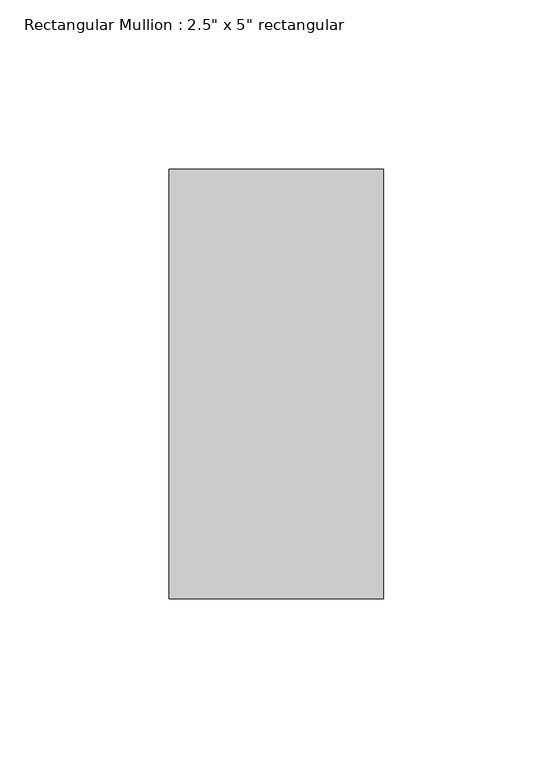
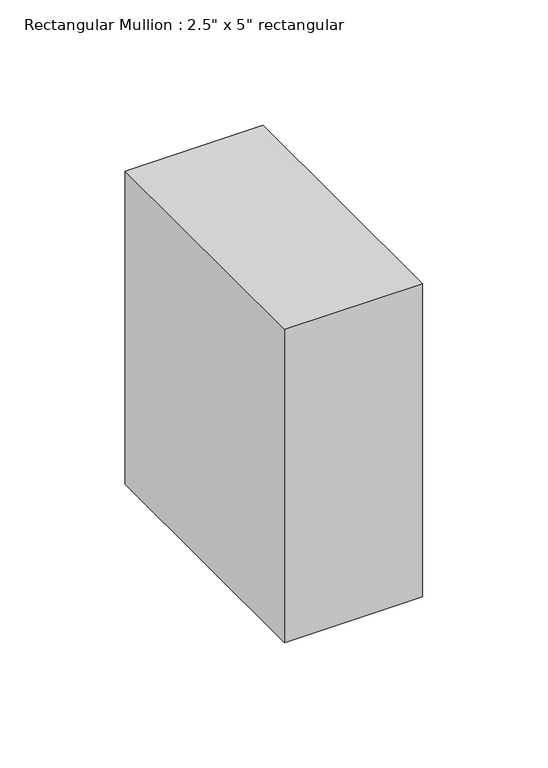
"""IFC4 building model written with IfcOpenShell, lengths in millimetres: member geometry."""

from ifc_helpers import new_model, si_unit, frame, origin, place, context, project, spatial, polyline, outline, extrude, source, transform, mapped, element, save


def member_876f8f00(model_context):
    return source(origin(), model_context, "Body", "SweptSolid", [
        extrude(outline(polyline([(0.0, 63.5), (0.0, -63.5), (-63.5, -63.5), (-63.5, 63.5), (0.0, 63.5)])), frame((0.0, 0.0, -152.4), z_axis=(0.0, 0.0, 1.0), x_axis=(1.0, 0.0, 0.0)), (0.0, 0.0, 1.0), 152.4),
    ])


if __name__ == "__main__":
    model = new_model("IFC4")
    model_context = context("Model", 3, world=origin())
    ifc_project = project(units=[si_unit("LENGTHUNIT", "METRE", prefix="MILLI")], contexts=[model_context])
    site = spatial("IfcSite", under=ifc_project)
    building = spatial("IfcBuilding", under=site)
    placement = place(None, origin())
    member_shape = member_876f8f00(model_context)
    element("IfcMember", 1, ObjectType="Rectangular Mullion : 2.5\" x 5\" rectangular", at=placement, inside=building, context=model_context, shape_type="MappedRepresentation", body=[
        mapped(member_shape, transform((0.0, 0.0, 0.0), x_axis=(1.0, 0.0, 0.0), y_axis=(0.0, 1.0, 0.0), z_axis=(0.0, 0.0, 1.0))),
    ])
    save(model, "model.ifc")

# Revit data of these elements
# Type "Rectangular Mullion : 2.5\" x 5\" rectangular"
#   built-in parameter 1007304 = 0.416667 (stored number, unit not read)
#   built-in parameter 1007301 = 0.104167 (stored number, unit not read)
#   built-in parameter 1007300 = 0.104167 (stored number, unit not read)
# Element 1 (IfcMember, "Rectangular Mullion : 2.5\" x 5\" rectangular")
#   Materials on its faces: "Aluminum"
# Materials
#   "Aluminum": class "Metal", colour RGB 247 247 247, transparency 0, Description = "Aluminum 6061", Cost = 0
